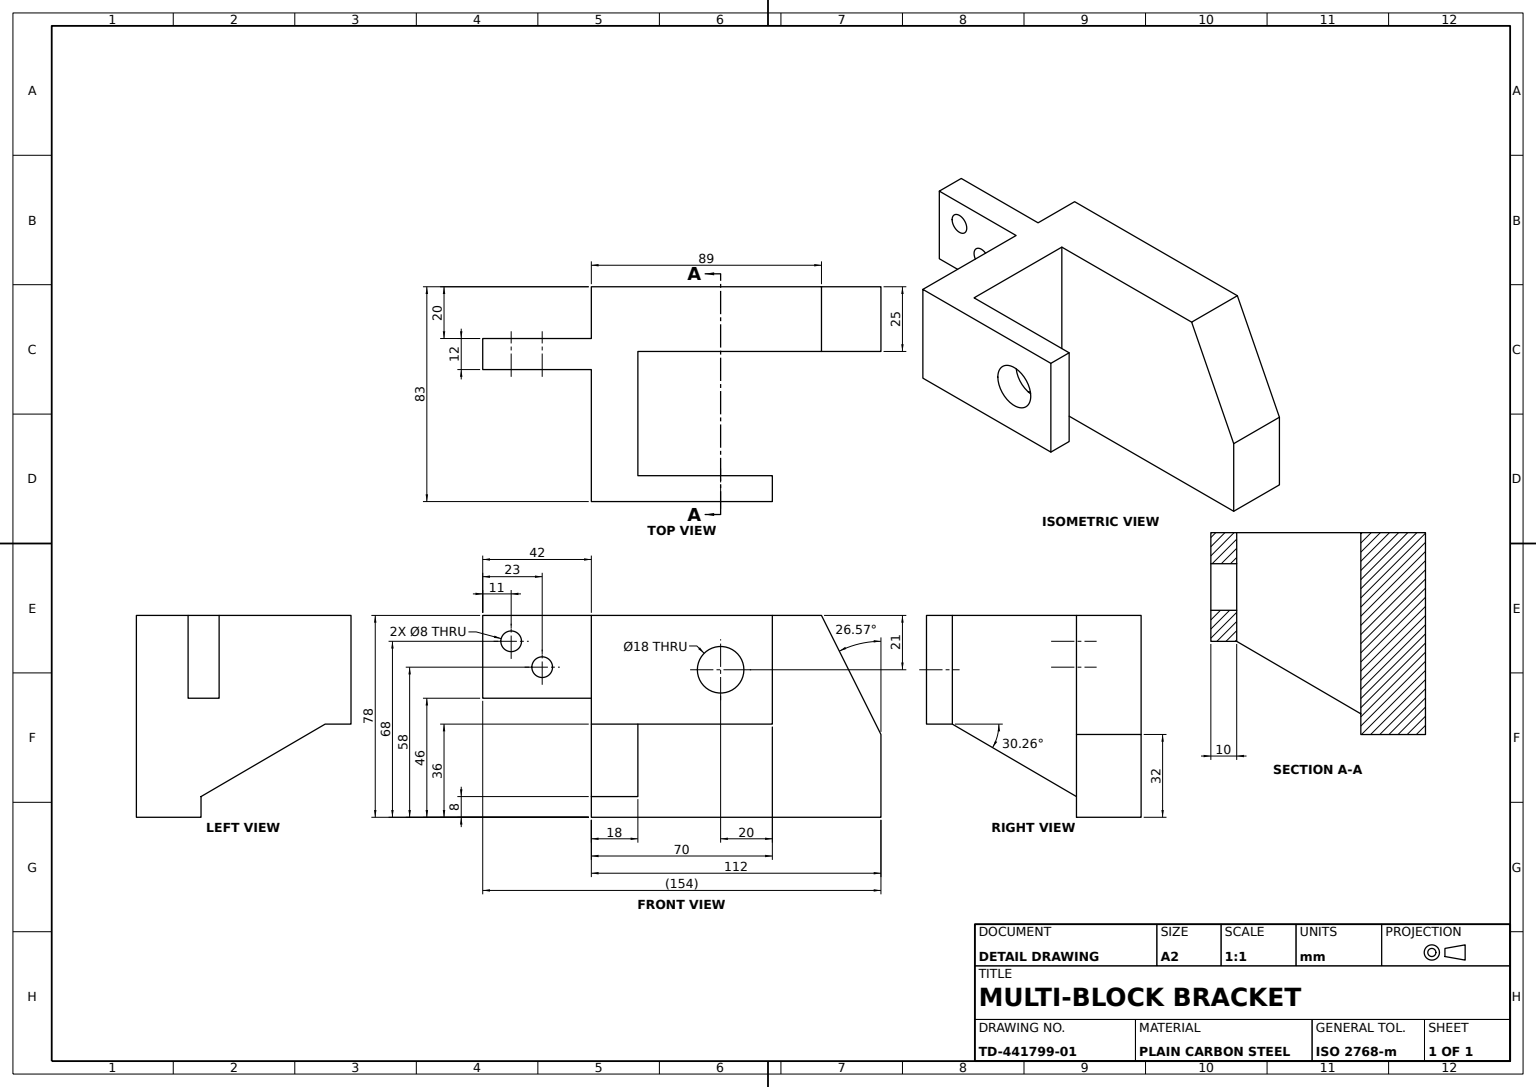
SolidWorks part; units mm, degrees
material "Plain Carbon Steel"
ref_plane "Front Plane" through (0, 0, 0) normal (0, 0, 1) x (1, 0, 0)
ref_plane "Top Plane" through (0, 0, 0) normal (0, 1, 0) x (1, 0, 0)
ref_plane "Right Plane" through (0, 0, 0) normal (1, 0, 0) x (0, 0, -1)
sketch "Base Block Sketch" plane through (0, 0, 0) normal (0, 0, 1) x (1, 0, 0)
  line L0 (0, 0) -> (112, 0)
  line L1 (0, 0) -> (0, 78)
  line L2 (112, 0) -> (112, 32)
  line L5 (0, 78) -> (89, 78)
  line L6 (89, 78) -> (112, 32)
  dimension "D1" = 89
  dimension "D2" = 112
  dimension "D3" = 32
  dimension "D4" = 78
extrude "Base Block" add sketch "Base Block Sketch" along normal blind 25
sketch "Upright Block Sketch" plane through (0, 0, 0) normal (-1, 0, 0) x (0, 0, 1)
  line L2 (71, 36) -> (25, 36)
  line L3 (25, 78) -> (25, 0) construction
  line L4 (25, 36) -> (25, 78)
  line L7 (25, 78) -> (83, 78)
  line L8 (83, 78) -> (83, 36)
  line L9 (83, 36) -> (71, 36)
  line L10 (0, 78) -> (0, 0) construction
  line L11 (25, 0) -> (0, 0) construction
  dimension "D1" = 71
  dimension "D2" = 83
  dimension "D3" = 36
extrude "Upright Block" add sketch "Upright Block Sketch" against normal blind 18
sketch "Side Tab Sketch" plane through (0, 0, 0) normal (-1, 0, 0) x (0, 0, 1)
  line L0 (0, 78) -> (0, 0) construction
  line L1 (83, 78) -> (0, 78) construction
  line L2 (20, 78) -> (20, 46)
  line L3 (20, 46) -> (32, 46)
  line L4 (32, 46) -> (32, 78)
  line L5 (32, 78) -> (20, 78)
  line L6 (25, 0) -> (0, 0) construction
  dimension "D1" = 20
  dimension "D2" = 32
  dimension "D3" = 46
extrude "Side Tab" add sketch "Side Tab Sketch" along normal blind 42
sketch "Front Plate Sketch" plane through (0, 0, 83) normal (0, 0, 1) x (1, 0, 0)
  line L0 (18, 78) -> (70, 78)
  line L1 (89, 78) -> (18, 78) construction
  line L2 (70, 78) -> (70, 36)
  line L3 (70, 36) -> (18, 36)
  line L4 (18, 36) -> (18, 78)
  line L5 (0, 36) -> (0, 78) construction
  dimension "D1" = 70
extrude "Front Plate" add sketch "Front Plate Sketch" against normal blind 10
sketch "Front Plate Hole Sketch" plane through (0, 0, 83) normal (0, 0, 1) x (1, 0, 0)
  line L0 (70, 36) -> (70, 78) construction
  line L1 (70, 78) -> (0, 78) construction
  circle A0 centre (50, 57) radius 9
  dimension "D1" = 18
  dimension "D4" = 18
  dimension "D2" = 20
  dimension "D3" = 21
extrude "Front Plate Hole" cut sketch "Front Plate Hole Sketch" against normal blind 10
sketch "Side Tab Holes Sketch" plane through (0, 0, 32) normal (0, 0, 1) x (1, 0, 0)
  line L0 (-42, 46) -> (-42, 78) construction
  line L1 (-42, 78) -> (0, 78) construction
  circle A0 centre (-31, 68) radius 4
  circle A1 centre (-19, 58) radius 4
  dimension "D1" = 8
  dimension "D4" = 8
  dimension "D7" = 8
  dimension "D2" = 11
  dimension "D3" = 10
  dimension "D5" = 23
  dimension "D6" = 20
extrude "Side Tab Holes 2x" cut sketch "Side Tab Holes Sketch" against normal blind 12
sketch "Gusset Sketch" plane through (0, 0, 0) normal (-1, 0, 0) x (0, 0, 1)
  line L0 (25, 36) -> (73, 36)
  line L3 (25, 36) -> (25, 0) construction
  line L4 (25, 8) -> (73, 36)
  line L6 (25, 8) -> (25, 36)
  line L8 (20, 78) -> (0, 78) construction
  dimension "D1" = 70
extrude "Triangular Gusset" add sketch "Gusset Sketch" against normal blind 18
